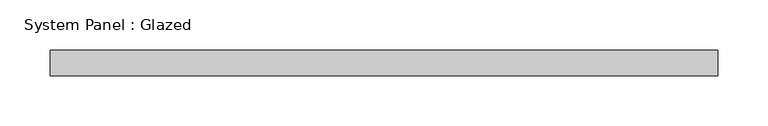
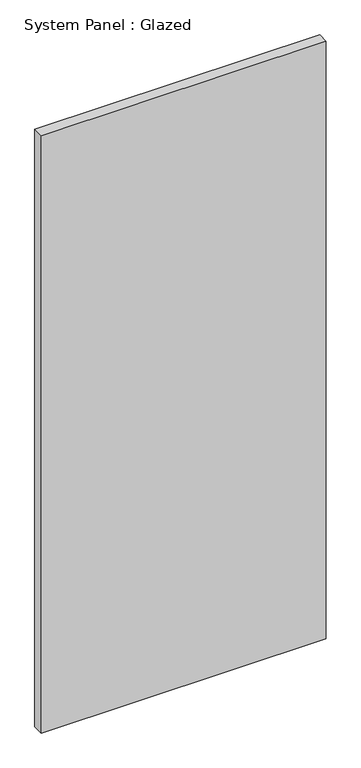
"""IFC4 building model written with IfcOpenShell, lengths in millimetres: plate geometry, System Panel : Glazed."""

from ifc_helpers import new_model, si_unit, origin, origin_with_axes, place, context, project, spatial, polyline, outline, extrude, source, transform, mapped, element, save


def system_panel_glazed_c0c7f1dd(model_context):
    return source(origin(), model_context, "Body", "SweptSolid", [
        extrude(outline(polyline([(333.375, 19.05), (-333.375, 19.05), (-333.375, 44.45), (333.375, 44.45), (333.375, 19.05)])), origin_with_axes(), (0.0, 0.0, 1.0), 1476.3915419),
    ])


if __name__ == "__main__":
    model = new_model("IFC4")
    model_context = context("Model", 3, world=origin())
    ifc_project = project(units=[si_unit("LENGTHUNIT", "METRE", prefix="MILLI")], contexts=[model_context])
    site = spatial("IfcSite", under=ifc_project)
    building = spatial("IfcBuilding", under=site)
    placement = place(None, origin())
    system_panel_glazed_shape = system_panel_glazed_c0c7f1dd(model_context)
    element("IfcPlate", 1, ObjectType="System Panel : Glazed", at=placement, inside=building, context=model_context, shape_type="MappedRepresentation", body=[
        mapped(system_panel_glazed_shape, transform((0.0, 0.0, 0.0), x_axis=(1.0, 0.0, 0.0), y_axis=(0.0, 1.0, 0.0), z_axis=(0.0, 0.0, 1.0))),
    ])
    save(model, "model.ifc")

# Revit data of these elements
# Type "System Panel : Glazed"
#   Construction Type Id = "GSP4R"
#   Analytic Construction = "1/8 in Pilkington single glazing"
#   Visual Light Transmittance = 0.9
#   Solar Heat Gain Coefficient = 0.86
#   Heat Transfer Coefficient (U) = 1.18115 BTU/(h·ft²·°F)
#   Define Thermal Properties by = 1
# Element 1 (IfcPlate, "System Panel : Glazed")
#   Materials on its faces: "Glass"
# Materials
#   "Glass": class "Glass", colour RGB 0 128 192, transparency 0.75, Description = "Soda Lime Glass", Cost = 0
